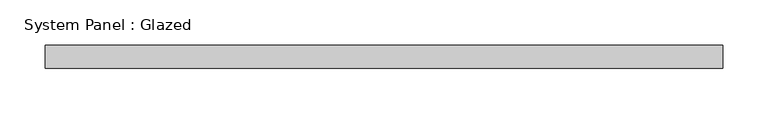
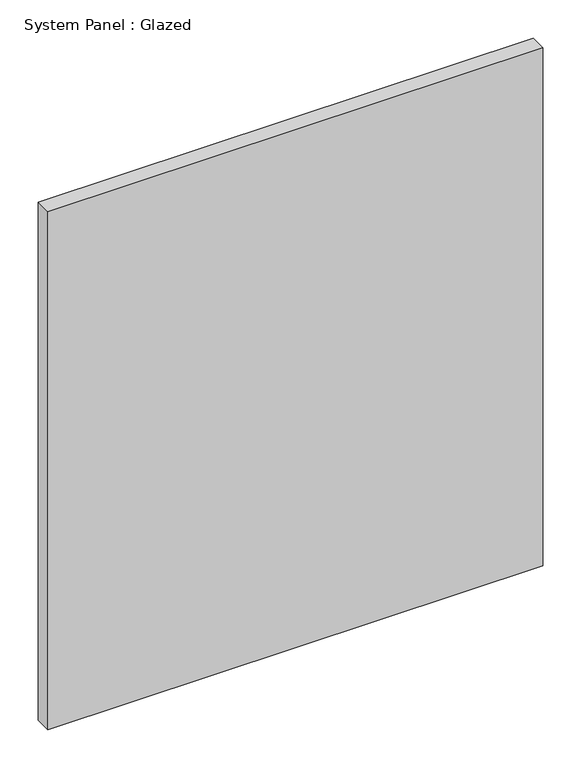
"""IFC4 building model written with IfcOpenShell, lengths in millimetres: plate geometry, System Panel : Glazed."""

from ifc_helpers import new_model, si_unit, origin, origin_with_axes, place, context, project, spatial, polyline, outline, extrude, source, transform, mapped, element, save


def system_panel_glazed_49caabb3(model_context):
    return source(origin(), model_context, "Body", "SweptSolid", [
        extrude(outline(polyline([(374.65, 19.05), (-374.65, 19.05), (-374.65, 44.45), (374.65, 44.45), (374.65, 19.05)])), origin_with_axes(), (0.0, 0.0, 1.0), 829.5094531),
    ])


if __name__ == "__main__":
    model = new_model("IFC4")
    model_context = context("Model", 3, world=origin())
    ifc_project = project(units=[si_unit("LENGTHUNIT", "METRE", prefix="MILLI")], contexts=[model_context])
    site = spatial("IfcSite", under=ifc_project)
    building = spatial("IfcBuilding", under=site)
    placement = place(None, origin())
    system_panel_glazed_shape = system_panel_glazed_49caabb3(model_context)
    element("IfcPlate", 1, ObjectType="System Panel : Glazed", at=placement, inside=building, context=model_context, shape_type="MappedRepresentation", body=[
        mapped(system_panel_glazed_shape, transform((0.0, 0.0, 0.0), x_axis=(1.0, 0.0, 0.0), y_axis=(0.0, 1.0, 0.0), z_axis=(0.0, 0.0, 1.0))),
    ])
    save(model, "model.ifc")

# Revit data of these elements
# Type "System Panel : Glazed"
#   Construction Type Id = "GSP4R"
#   Analytic Construction = "1/8 in Pilkington single glazing"
#   Visual Light Transmittance = 0.9
#   Solar Heat Gain Coefficient = 0.86
#   Heat Transfer Coefficient (U) = 1.18115 BTU/(h·ft²·°F)
#   Define Thermal Properties by = 1
# Element 1 (IfcPlate, "System Panel : Glazed")
#   Materials on its faces: "Glass"
# Materials
#   "Glass": class "Glass", colour RGB 0 128 192, transparency 0.75, Description = "Soda Lime Glass", Cost = 0
